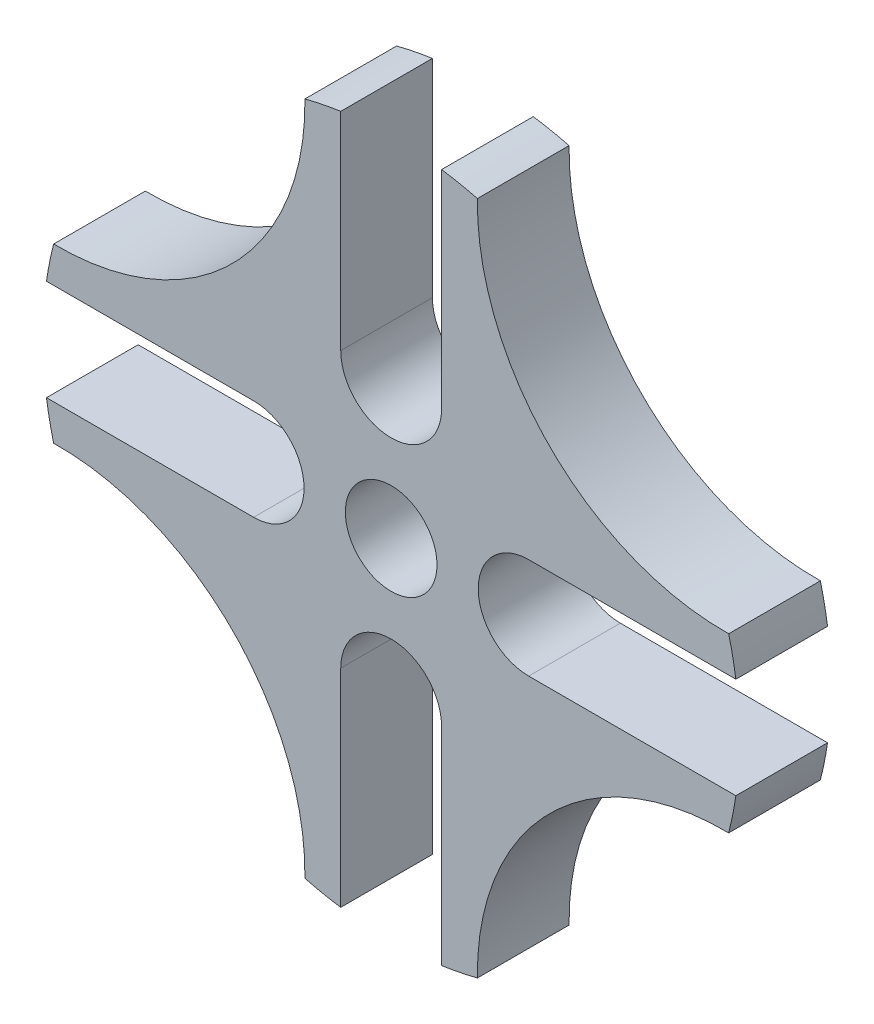
SolidWorks part; units mm, degrees
material "Plain Carbon Steel"
ref_plane "Front Plane" through (0, 0, 0) normal (0, 0, 1) x (1, 0, 0)
ref_plane "Top Plane" through (0, 0, 0) normal (0, 1, 0) x (1, 0, 0)
ref_plane "Right Plane" through (0, 0, 0) normal (1, 0, 0) x (0, 0, -1)
sketch "Spider Plate Profile" plane through (0, 0, 0) normal (0, 0, 1) x (1, 0, 0)
  line L0 (0, 0) -> (38.2, 0) construction
  line L1 (5.5, -15) -> (5.5, -37.5999)
  line L2 (-5.5, -15) -> (-5.5, -37.5999)
  line L3 (-15, -5.5) -> (-37.5999, -5.5)
  line L4 (-15, 5.5) -> (-37.5999, 5.5)
  line L5 (-5.5, 15) -> (-5.5, 37.5999)
  line L6 (5.5, 15) -> (5.5, 37.5999)
  line L7 (15, 5.5) -> (37.5999, 5.5)
  line L8 (15, -5.5) -> (37.5999, -5.5)
  line L9 (0, 0) -> (36.9535, 36.9535) construction
  circle A0 centre (0, 0) radius 5
  arc A1 (5.5, -37.5999) -> (9.4083, -36.8169) centre (0, 0) ccw
  arc A2 (5.5, -15) -> (-5.5, -15) centre (0, -15) ccw
  arc A3 (-15, -5.5) -> (-15, 5.5) centre (-15, 0) ccw
  arc A4 (-5.5, 15) -> (5.5, 15) centre (0, 15) ccw
  arc A5 (15, 5.5) -> (15, -5.5) centre (15, 0) ccw
  arc A6 (9.4083, 36.8169) -> (36.8169, 9.4083) centre (36.4051, 36.4051) ccw
  arc A7 (36.8169, -9.4083) -> (9.4083, -36.8169) centre (36.4051, -36.4051) ccw
  arc A8 (-9.4083, -36.8169) -> (-36.8169, -9.4083) centre (-36.4051, -36.4051) ccw
  arc A9 (-36.8169, 9.4083) -> (-9.4083, 36.8169) centre (-36.4051, 36.4051) ccw
  arc A10 (37.5999, 5.5) -> (36.8169, 9.4083) centre (0, 0) ccw
  arc A11 (-5.5, 37.5999) -> (-9.4083, 36.8169) centre (0, 0) ccw
  arc A12 (-37.5999, -5.5) -> (-36.8169, -9.4083) centre (0, 0) ccw
  arc A13 (-9.4083, -36.8169) -> (-5.5, -37.5999) centre (0, 0) ccw
  arc A14 (36.8169, -9.4083) -> (37.5999, -5.5) centre (0, 0) ccw
  arc A15 (9.4083, 36.8169) -> (5.5, 37.5999) centre (0, 0) ccw
  arc A16 (-36.8169, 9.4083) -> (-37.5999, 5.5) centre (0, 0) ccw
  point P28 (0, 0)
  point P42 (0, 0)
  dimension "D1" = 10
  dimension "D3" = 76
  dimension "D4" = 11
  dimension "D8" = 27
  dimension "D2" = 38.2
  dimension "D5" = 15
  dimension "D7" = 45
  dimension "D10" = 14.9083
  dimension "D6" = 4
  dimension "D9" = 4
extrude "Spider Plate Extrude 10mm" add sketch "Spider Plate Profile" along normal blind 10
